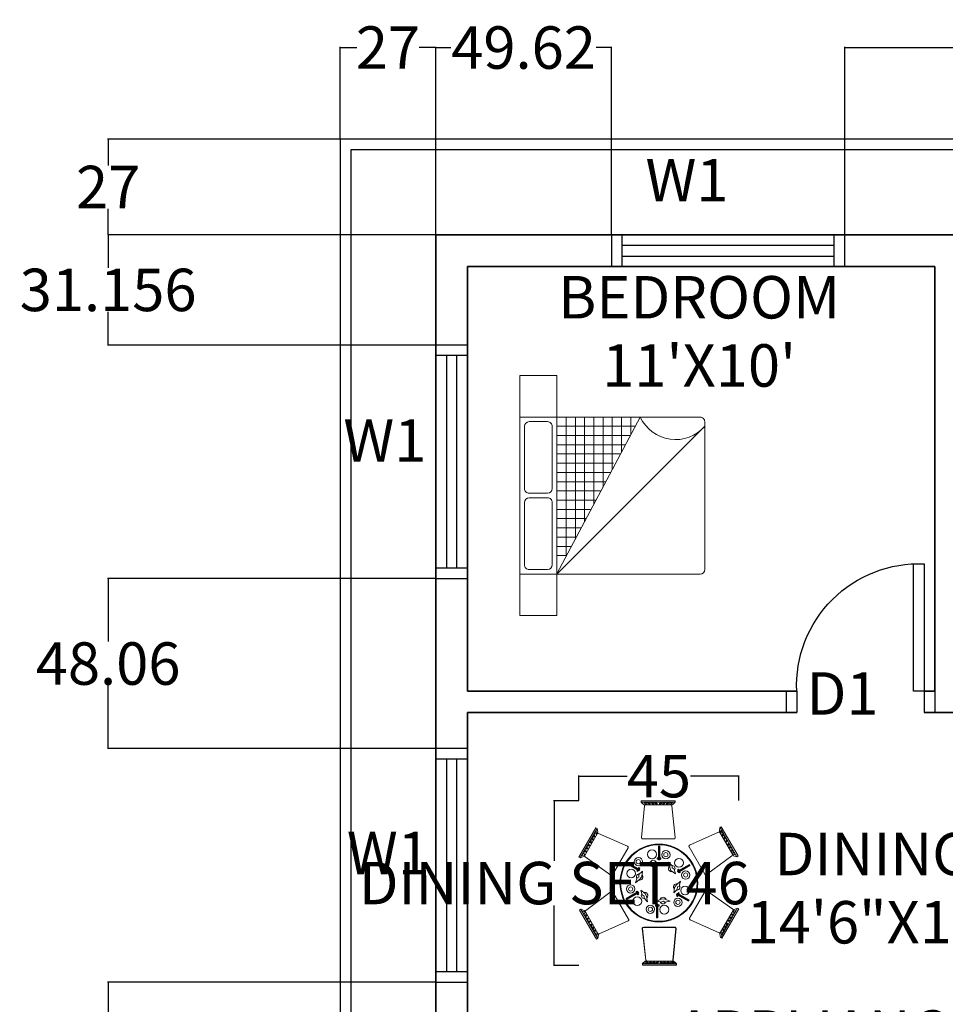
# Model space of a CAD drawing. Units: inches. Extents: x 774 to 1314, y 374 to 930.
# Tile 4 of 5: x 774 to 1035, y 652 to 930. Entities that reach past the tile are written whole.
import ezdxf
from ezdxf.enums import TextEntityAlignment as Align

# ---------------------------------------------------------------- set-up
doc = ezdxf.new("R2010")
doc.units = ezdxf.units.IN
doc.header["$MEASUREMENT"] = 0
for name, color, linetype, lineweight in [('A-ANNO-DIMS', 2, 'Continuous', 18), ('A-ANNO-TEXT', 2, 'Continuous', 18), ('A-AREA-IDEN', 2, 'Continuous', 18), ('A-DOOR', 6, 'Continuous', 25), ('A-FURN', 8, 'Continuous', 18), ('A-GLAZ', 4, 'Continuous', 18), ('A-WALL', 1, 'Continuous', 35), ('C-PROP', 3, 'Continuous', 25)]:
    doc.layers.add(name, color=color, linetype=linetype, lineweight=lineweight)
doc.layers.add('Layer4', color=4, linetype='Continuous')
doc.styles.get("Standard").update_dxf_attribs({"font": 'arial.ttf'})
doc.dimstyles.get("Standard").update_dxf_attribs({"dimtxt": 12, "dimasz": 0.18, "dimexe": 0.18, "dimexo": 0.0625, "dimgap": 0.09, "dimtad": 0, "dimtih": 1, "dimtoh": 1, "dimdec": 0, "dimzin": 0, "dimdsep": 46, "dimlunit": 4, "dimtxsty": 'Standard', "dimcen": 0.09, "dimadec": 0, "dimazin": 0, "dimtfac": 1, "dimtdec": 0, "dimtofl": 0, "dimtmove": 0, "dimatfit": 3, "dimfxl": 1, "dimtolj": 1, "dimtzin": 0, "dimarcsym": 0})

# ---------------------------------------------------------------- blocks, each defined once
blk = doc.blocks.new('tr')
at = {"layer": 'Layer4'}
for p, q in [((9, 66), (0, 66)), ((9, 63), (0, 63)), ((0, 63), (0, 3)), ((3, 63), (3, 3)), ((6, 3), (6, 63)), ((9, 3), (9, 63)), ((0, 3), (9, 3)), ((0, 0), (9, 0))]:
    blk.add_line(p, q, dxfattribs=at)
blk = doc.blocks.new('A$C45501D90')
for p, q in [((-242, 1134), (224, 1134)), ((-242, 1113), (-242, 1134)), ((224, 1113), (-242, 1113)), ((-242, 1111), (-202, 1079)), ((-204, 1106), (-166, 1108)), ((-169, 1081), (-204, 1106)), ((-166, 1108), (-167, 1086)), ((-156, 1110), (-132, 1086)), ((-119, 1086), (-143, 1108)), ((-143, 1108), (-134, 1108)), ((-134, 1108), (-122, 1098)), ((-122, 1098), (-119, 1102)), ((-119, 1102), (-118, 1087)), ((-108, 1110), (-84, 1086)), ((-71, 1086), (-95, 1108)), ((-95, 1108), (-86, 1108)), ((-86, 1108), (-75, 1098)), ((-75, 1098), (-71, 1102)), ((-71, 1102), (-70, 1087)), ((-60, 1110), (-36, 1086)), ((-23, 1086), (-47, 1108)), ((-47, 1108), (-38, 1108)), ((-38, 1108), (-27, 1098)), ((-27, 1098), (-23, 1102)), ((-23, 1102), (-22, 1087)), ((8, 1102), (7, 1087)), ((8, 1086), (32, 1108)), ((12, 1098), (8, 1102)), ((23, 1108), (12, 1098)), ((45, 1110), (21, 1086)), ((32, 1108), (23, 1108)), ((56, 1102), (55, 1087)), ((56, 1086), (80, 1108)), ((60, 1098), (56, 1102)), ((71, 1108), (60, 1098)), ((93, 1110), (69, 1086)), ((80, 1108), (71, 1108)), ((104, 1102), (103, 1087)), ((104, 1086), (128, 1108)), ((107, 1098), (104, 1102)), ((119, 1108), (107, 1098)), ((141, 1110), (117, 1086)), ((128, 1108), (119, 1108)), ((189, 1106), (151, 1108)), ((151, 1108), (152, 1086)), ((154, 1081), (189, 1106)), ((224, 1113), (187, 1079)), ((224, 1134), (224, 1113)), ((-197, 1062), (-239, 628)), ((-202, 1079), (-169, 1081)), ((162, 1076), (-181, 1076)), ((-132, 1086), (-119, 1086)), ((-84, 1086), (-71, 1086)), ((-36, 1086), (-23, 1086)), ((21, 1086), (8, 1086)), ((69, 1086), (56, 1086)), ((117, 1086), (104, 1086)), ((187, 1079), (154, 1081)), ((225, 628), (178, 1062)), ((-1103, 357), (-870, 761)), ((-852, 750), (-1085, 347)), ((-864, 717), (-884, 684)), ((-884, 684), (-864, 675)), ((-870, 761), (-852, 750)), ((-859, 674), (-864, 717)), ((-841, 702), (-859, 674)), ((-849, 752), (-841, 702)), ((-431, 509), (-831, 685)), ((821, 702), (424, 521)), ((841, 765), (834, 715)), ((834, 715), (852, 687)), ((1013, 398), (841, 695)), ((843, 766), (861, 776)), ((1076, 362), (843, 766)), ((852, 687), (856, 730)), ((856, 730), (877, 697)), ((877, 697), (857, 688)), ((861, 776), (1094, 373)), ((883, 690), (874, 657)), ((-851, 678), (-1023, 381)), ((-945, 559), (-950, 558)), ((-950, 558), (-938, 550)), ((-943, 582), (-948, 574)), ((-948, 574), (-945, 559)), ((-936, 550), (-943, 582)), ((-938, 594), (-930, 561)), ((-930, 561), (-936, 550)), ((-921, 601), (-926, 600)), ((-926, 600), (-914, 591)), ((-919, 624), (-924, 615)), ((-924, 615), (-921, 601)), ((-912, 592), (-919, 624)), ((-914, 635), (-906, 603)), ((-906, 603), (-912, 592)), ((-898, 642), (-902, 641)), ((-902, 641), (-890, 633)), ((-895, 665), (-900, 657)), ((-900, 657), (-898, 642)), ((-888, 633), (-895, 665)), ((-890, 677), (-882, 644)), ((-882, 644), (-888, 633)), ((-223, 610), (209, 610)), ((874, 657), (881, 646)), ((881, 646), (888, 678)), ((894, 654), (883, 646)), ((888, 678), (893, 670)), ((893, 670), (890, 655)), ((890, 655), (894, 654)), ((907, 648), (898, 616)), ((898, 616), (904, 605)), ((904, 605), (912, 637)), ((918, 613), (907, 604)), ((912, 637), (917, 628)), ((917, 628), (914, 614)), ((914, 614), (918, 613)), ((931, 607), (922, 574)), ((922, 574), (928, 563)), ((928, 563), (936, 595)), ((942, 571), (931, 563)), ((936, 595), (941, 587)), ((941, 587), (938, 572)), ((938, 572), (942, 571)), ((958, 543), (945, 538)), ((957, 539), (958, 543)), ((-1060, 377), (-1042, 411)), ((-1042, 411), (-1024, 398)), ((-1039, 420), (-1006, 428)), ((-1000, 440), (-1031, 430)), ((-1031, 430), (-1026, 438)), ((-1026, 438), (-1012, 443)), ((-1015, 461), (-982, 470)), ((-1012, 443), (-1014, 448)), ((-1014, 448), (-1000, 442)), ((-976, 481), (-1007, 471)), ((-1007, 471), (-1002, 480)), ((-1006, 428), (-1000, 440)), ((-1002, 480), (-989, 485)), ((-991, 503), (-958, 511)), ((-989, 485), (-990, 489)), ((-990, 489), (-976, 483)), ((-952, 522), (-983, 513)), ((-983, 513), (-978, 521)), ((-982, 470), (-976, 481)), ((-978, 521), (-965, 526)), ((-965, 526), (-966, 530)), ((-966, 530), (-953, 525)), ((-958, 511), (-952, 522)), ((-640, 112), (-424, 486)), ((-6, 509, 91), (0, 509, 91)), ((-6, 318, 91), (-6, 509, 91)), ((0, 509, 91), (0, 318, 91)), ((6, 318, 91), (6, 509, 91)), ((6, 509, 91), (12, 509, 91)), ((12, 509, 91), (12, 318, 91)), ((417, 498), (633, 124)), ((951, 524), (944, 535)), ((944, 535), (976, 526)), ((983, 516), (951, 524)), ((971, 534), (957, 539)), ((968, 494), (1000, 484)), ((975, 483), (968, 494)), ((982, 502), (969, 496)), ((976, 526), (971, 534)), ((1007, 474), (975, 483)), ((981, 498), (982, 502)), ((995, 493), (981, 498)), ((999, 441), (992, 453)), ((992, 453), (1024, 443)), ((1006, 461), (993, 455)), ((1000, 484), (995, 493)), ((1031, 433), (999, 441)), ((1005, 456), (1006, 461)), ((1019, 451), (1005, 456)), ((1035, 424), (1016, 411)), ((1024, 443), (1019, 451)), ((1053, 390), (1035, 424)), ((-1085, 347), (-1103, 357)), ((-1083, 346), (-1036, 364)), ((-1020, 394), (-1060, 377)), ((-1036, 364), (-1020, 394)), ((-1018, 360), (-663, 107)), ((-431, 275, 91), (-428, 280, 91)), ((-265, 180, 91), (-431, 275, 91)), ((-428, 280, 91), (-262, 185, 91)), ((-175, 276, 91), (-105, 293, 91)), ((-103, 252, 91), (-175, 276, 91)), ((-105, 293, 91), (-86, 278, 91)), ((-86, 278, 91), (-52, 294, 91)), ((9, 276, 91), (-60, 246, 91)), ((-52, 294, 91), (9, 276, 91)), ((-22, 329, 91), (-22, 345, 91)), ((-22, 345, 91), (-6, 345, 91)), ((-6, 329, 91), (-22, 329, 91)), ((0, 318, 91), (-6, 318, 91)), ((0, 345, 91), (6, 345, 91)), ((6, 329, 91), (0, 329, 91)), ((12, 318, 91), (6, 318, 91)), ((12, 345, 91), (27, 345, 91)), ((27, 329, 91), (12, 329, 91)), ((27, 345, 91), (27, 329, 91)), ((134, 288, 91), (184, 236, 91)), ((150, 214, 91), (134, 288, 91)), ((656, 119), (1008, 377)), ((1028, 377), (1013, 407)), ((1013, 407), (1053, 390)), ((1076, 359), (1028, 377)), ((1094, 373), (1076, 362)), ((-436, 265, 91), (-433, 271, 91)), ((-271, 170, 91), (-436, 265, 91)), ((-433, 271, 91), (-268, 175, 91)), ((-303, 169, 91), (-294, 183, 91)), ((-289, 161, 91), (-303, 169, 91)), ((-291, 188, 91), (-289, 193, 91)), ((-281, 176, 91), (-289, 161, 91)), ((-286, 198, 91), (-278, 212, 91)), ((-278, 212, 91), (-264, 204, 91)), ((-275, 185, 91), (-278, 181, 91)), ((-274, 118, 91), (-227, 162, 91)), ((-264, 204, 91), (-272, 191, 91)), ((-268, 175, 91), (-271, 170, 91)), ((-262, 185, 91), (-265, 180, 91)), ((-227, 162, 91), (-236, 87, 91)), ((-60, 246, 91), (-103, 252, 91)), ((166, 173, 91), (150, 214, 91)), ((227, 128, 91), (166, 173, 91)), ((184, 236, 91), (181, 211, 91)), ((181, 211, 91), (211, 190, 91)), ((211, 190, 91), (227, 128, 91)), ((255, 162, 91), (421, 257, 91)), ((258, 157, 91), (255, 162, 91)), ((257, 182, 91), (270, 190, 91)), ((265, 168, 91), (257, 182, 91)), ((424, 252, 91), (258, 157, 91)), ((261, 152, 91), (426, 248, 91)), ((264, 147, 91), (261, 152, 91)), ((429, 242, 91), (264, 147, 91)), ((271, 158, 91), (268, 162, 91)), ((270, 190, 91), (278, 175, 91)), ((281, 139, 91), (274, 153, 91)), ((281, 170, 91), (284, 165, 91)), ((295, 147, 91), (281, 139, 91)), ((287, 160, 91), (295, 147, 91)), ((421, 257, 91), (424, 252, 91)), ((426, 248, 91), (429, 242, 91)), ((-320, 2, 91), (-299, 72, 91)), ((-263, 53, 91), (-320, 2, 91)), ((-299, 72, 91), (-277, 81, 91)), ((-277, 81, 91), (-274, 118, 91)), ((-236, 87, 91), (-263, 53, 91)), ((243, -25, 91), (299, 26, 91)), ((299, 26, 91), (279, -44, 91)), ((-656, -119), (-1008, -377)), ((-417, -498), (-633, -124)), ((-450, -214, 91), (-284, -119, 91)), ((-281, -124, 91), (-447, -220, 91)), ((-444, -224, 91), (-279, -129, 91)), ((-276, -134, 91), (-441, -229, 91)), ((-315, -119, 91), (-302, -111, 91)), ((-307, -132, 91), (-315, -119, 91)), ((-302, -111, 91), (-294, -125, 91)), ((-291, -130, 91), (-288, -134, 91)), ((-284, -119, 91), (-281, -124, 91)), ((-279, -129, 91), (-276, -134, 91)), ((-247, -100, 91), (-187, -145, 91)), ((-232, -162, 91), (-247, -100, 91)), ((207, -134, 91), (216, -60, 91)), ((253, -90, 91), (207, -134, 91)), ((216, -60, 91), (243, -25, 91)), ((256, -53, 91), (253, -90, 91)), ((279, -44, 91), (256, -53, 91)), ((260, -148, 91), (269, -133, 91)), ((269, -133, 91), (282, -141, 91)), ((640, -112), (424, -486)), ((1018, -360), (663, -107)), ((-447, -220, 91), (-450, -214, 91)), ((-441, -229, 91), (-444, -224, 91)), ((-302, -142, 91), (-304, -137, 91)), ((-290, -162, 91), (-299, -147, 91)), ((-277, -154, 91), (-290, -162, 91)), ((-285, -140, 91), (-277, -154, 91)), ((-201, -183, 91), (-232, -162, 91)), ((-205, -208, 91), (-201, -183, 91)), ((-155, -260, 91), (-205, -208, 91)), ((-187, -145, 91), (-170, -186, 91)), ((-170, -186, 91), (-155, -260, 91)), ((-30, -248, 91), (39, -218, 91)), ((32, -266, 91), (-30, -248, 91)), ((65, -250, 91), (32, -266, 91)), ((39, -218, 91), (83, -224, 91)), ((84, -265, 91), (65, -250, 91)), ((83, -224, 91), (155, -248, 91)), ((155, -248, 91), (84, -265, 91)), ((242, -157, 91), (245, -152, 91)), ((407, -252, 91), (242, -157, 91)), ((244, -176, 91), (252, -163, 91)), ((257, -184, 91), (244, -176, 91)), ((245, -152, 91), (410, -247, 91)), ((248, -147, 91), (251, -142, 91)), ((413, -243, 91), (248, -147, 91)), ((251, -142, 91), (416, -237, 91)), ((255, -157, 91), (257, -153, 91)), ((265, -170, 91), (257, -184, 91)), ((271, -160, 91), (268, -165, 91)), ((282, -141, 91), (274, -155, 91)), ((410, -247, 91), (407, -252, 91)), ((416, -237, 91), (413, -243, 91)), ((-1094, -373), (-1076, -362)), ((-861, -776), (-1094, -373)), ((-1076, -359), (-1028, -377)), ((-1076, -362), (-843, -766)), ((-1053, -390), (-1035, -424)), ((-1013, -407), (-1053, -390)), ((-1028, -377), (-1013, -407)), ((-1013, -398), (-841, -695)), ((-48, -317, 91), (-48, -301, 91)), ((-48, -301, 91), (-32, -301, 91)), ((-32, -317, 91), (-48, -317, 91)), ((-32, -481, 91), (-32, -290, 91)), ((-32, -290, 91), (-26, -290, 91)), ((-26, -290, 91), (-26, -481, 91)), ((-26, -301, 91), (-21, -301, 91)), ((-21, -317, 91), (-26, -317, 91)), ((-21, -481, 91), (-21, -290, 91)), ((-21, -290, 91), (-15, -290, 91)), ((-15, -290, 91), (-15, -481, 91)), ((-15, -301, 91), (2, -301, 91)), ((2, -317, 91), (-15, -317, 91)), ((2, -301, 91), (2, -317, 91)), ((851, -678), (1023, -381)), ((852, -750), (1085, -347)), ((1103, -357), (870, -761)), ((1036, -364), (1020, -394)), ((1020, -394), (1060, -377)), ((1042, -411), (1024, -398)), ((1083, -346), (1036, -364)), ((1060, -377), (1042, -411)), ((1085, -347), (1103, -357)), ((-1035, -424), (-1016, -411)), ((-1031, -433), (-999, -441)), ((-1024, -443), (-1019, -451)), ((-992, -453), (-1024, -443)), ((-1019, -451), (-1005, -456)), ((-1007, -474), (-975, -483)), ((-1006, -461), (-993, -455)), ((-1005, -456), (-1006, -461)), ((-968, -494), (-1000, -484)), ((-1000, -484), (-995, -493)), ((-999, -441), (-992, -453)), ((-995, -493), (-981, -498)), ((-983, -516), (-951, -524)), ((-982, -502), (-969, -496)), ((-981, -498), (-982, -502)), ((-944, -535), (-976, -526)), ((-976, -526), (-971, -534)), ((-975, -483), (-968, -494)), ((-971, -534), (-957, -539)), ((-958, -543), (-945, -538)), ((-957, -539), (-958, -543)), ((-951, -524), (-944, -535)), ((-821, -702), (-424, -521)), ((-26, -481, 91), (-32, -481, 91)), ((-15, -481, 91), (-21, -481, 91)), ((431, -509), (831, -685)), ((958, -511), (952, -522)), ((952, -522), (983, -513)), ((966, -530), (953, -525)), ((991, -503), (958, -511)), ((978, -521), (965, -526)), ((965, -526), (966, -530)), ((982, -470), (976, -481)), ((976, -481), (1007, -471)), ((990, -489), (976, -483)), ((983, -513), (978, -521)), ((1015, -461), (982, -470)), ((1002, -480), (989, -485)), ((989, -485), (990, -489)), ((1006, -428), (1000, -440)), ((1000, -440), (1031, -430)), ((1014, -448), (1000, -442)), ((1007, -471), (1002, -480)), ((1039, -420), (1006, -428)), ((1026, -438), (1012, -443)), ((1012, -443), (1014, -448)), ((1031, -430), (1026, -438)), ((-942, -571), (-931, -563)), ((-938, -572), (-942, -571)), ((-941, -587), (-938, -572)), ((-936, -595), (-941, -587)), ((-928, -563), (-936, -595)), ((-931, -607), (-922, -574)), ((-922, -574), (-928, -563)), ((-918, -613), (-907, -604)), ((-914, -614), (-918, -613)), ((-917, -628), (-914, -614)), ((-912, -637), (-917, -628)), ((-904, -605), (-912, -637)), ((-907, -648), (-898, -616)), ((-898, -616), (-904, -605)), ((-894, -654), (-883, -646)), ((-890, -655), (-894, -654)), ((-893, -670), (-890, -655)), ((-888, -678), (-893, -670)), ((-881, -646), (-888, -678)), ((-883, -690), (-874, -657)), ((-874, -657), (-881, -646)), ((-229, -629), (-182, -1063)), ((-225, -628), (-178, -1062)), ((219, -612), (-213, -612)), ((223, -610), (-209, -610)), ((193, -1063), (235, -629)), ((197, -1062), (239, -628)), ((841, -702), (859, -674)), ((859, -674), (864, -717)), ((884, -684), (864, -675)), ((882, -644), (888, -633)), ((890, -677), (882, -644)), ((888, -633), (895, -665)), ((902, -641), (890, -633)), ((895, -665), (900, -657)), ((898, -642), (902, -641)), ((900, -657), (898, -642)), ((906, -603), (912, -592)), ((914, -635), (906, -603)), ((912, -592), (919, -624)), ((926, -600), (914, -591)), ((919, -624), (924, -615)), ((921, -601), (926, -600)), ((924, -615), (921, -601)), ((930, -561), (936, -550)), ((938, -594), (930, -561)), ((936, -550), (943, -582)), ((950, -558), (938, -550)), ((943, -582), (948, -574)), ((945, -559), (950, -558)), ((948, -574), (945, -559)), ((-877, -697), (-857, -688)), ((-856, -730), (-877, -697)), ((-843, -766), (-861, -776)), ((-852, -687), (-856, -730)), ((-834, -715), (-852, -687)), ((-841, -765), (-834, -715)), ((849, -752), (841, -702)), ((870, -761), (852, -750)), ((864, -717), (884, -684)), ((-231, -1113), (-191, -1081)), ((-227, -1111), (-187, -1079)), ((-158, -1082), (-193, -1108)), ((-191, -1081), (-158, -1082)), ((-154, -1081), (-189, -1106)), ((-187, -1079), (-154, -1081)), ((-166, -1078), (177, -1078)), ((-162, -1076), (181, -1076)), ((-151, -1108), (-152, -1086)), ((-141, -1110), (-117, -1086)), ((-104, -1086), (-128, -1108)), ((-117, -1086), (-104, -1086)), ((-93, -1110), (-69, -1086)), ((-56, -1086), (-80, -1108)), ((-69, -1086), (-56, -1086)), ((-45, -1110), (-21, -1086)), ((-8, -1086), (-32, -1108)), ((-21, -1086), (-8, -1086)), ((23, -1086), (47, -1108)), ((36, -1086), (23, -1086)), ((60, -1110), (36, -1086)), ((71, -1086), (95, -1108)), ((84, -1086), (71, -1086)), ((108, -1110), (84, -1086)), ((119, -1086), (143, -1108)), ((132, -1086), (119, -1086)), ((156, -1110), (132, -1086)), ((198, -1081), (165, -1082)), ((165, -1082), (200, -1108)), ((166, -1108), (167, -1086)), ((202, -1079), (169, -1081)), ((169, -1081), (204, -1106)), ((238, -1113), (198, -1081)), ((242, -1111), (202, -1079)), ((-228, -1114), (238, -1114)), ((-228, -1135), (-228, -1114)), ((238, -1135), (-228, -1135)), ((-224, -1113), (242, -1113)), ((-224, -1134), (-224, -1113)), ((242, -1134), (-224, -1134)), ((-193, -1108), (-155, -1109)), ((-189, -1106), (-151, -1108)), ((-155, -1109), (-156, -1087)), ((-145, -1111), (-121, -1087)), ((-108, -1087), (-132, -1109)), ((-132, -1109), (-123, -1109)), ((-128, -1108), (-119, -1108)), ((-123, -1109), (-112, -1100)), ((-121, -1087), (-108, -1087)), ((-119, -1108), (-107, -1098)), ((-112, -1100), (-108, -1103)), ((-108, -1103), (-107, -1089)), ((-107, -1098), (-104, -1102)), ((-104, -1102), (-103, -1087)), ((-97, -1111), (-73, -1087)), ((-60, -1087), (-84, -1109)), ((-84, -1109), (-75, -1109)), ((-80, -1108), (-71, -1108)), ((-75, -1109), (-64, -1100)), ((-73, -1087), (-60, -1087)), ((-71, -1108), (-60, -1098)), ((-64, -1100), (-60, -1103)), ((-60, -1103), (-59, -1089)), ((-60, -1098), (-56, -1102)), ((-56, -1102), (-55, -1087)), ((-49, -1111), (-25, -1087)), ((-13, -1087), (-37, -1109)), ((-37, -1109), (-27, -1109)), ((-32, -1108), (-23, -1108)), ((-27, -1109), (-16, -1100)), ((-25, -1087), (-13, -1087)), ((-23, -1108), (-12, -1098)), ((-16, -1100), (-13, -1103)), ((-13, -1103), (-11, -1089)), ((-12, -1098), (-8, -1102)), ((-8, -1102), (-7, -1087)), ((19, -1103), (18, -1089)), ((19, -1087), (43, -1109)), ((32, -1087), (19, -1087)), ((23, -1100), (19, -1103)), ((23, -1102), (22, -1087)), ((27, -1098), (23, -1102)), ((34, -1109), (23, -1100)), ((38, -1108), (27, -1098)), ((56, -1111), (32, -1087)), ((43, -1109), (34, -1109)), ((47, -1108), (38, -1108)), ((67, -1103), (66, -1089)), ((67, -1087), (91, -1109)), ((80, -1087), (67, -1087)), ((70, -1100), (67, -1103)), ((71, -1102), (70, -1087)), ((82, -1109), (70, -1100)), ((75, -1098), (71, -1102)), ((86, -1108), (75, -1098)), ((104, -1111), (80, -1087)), ((91, -1109), (82, -1109)), ((95, -1108), (86, -1108)), ((115, -1103), (114, -1089)), ((115, -1087), (139, -1109)), ((128, -1087), (115, -1087)), ((118, -1100), (115, -1103)), ((119, -1102), (118, -1087)), ((130, -1109), (118, -1100)), ((122, -1098), (119, -1102)), ((134, -1108), (122, -1098)), ((152, -1111), (128, -1087)), ((139, -1109), (130, -1109)), ((143, -1108), (134, -1108)), ((161, -1109), (163, -1087)), ((200, -1108), (161, -1109)), ((204, -1106), (166, -1108)), ((238, -1114), (238, -1135)), ((242, -1113), (242, -1134))]:
    blk.add_line(p, q)
for centre, radius in [((0, 0), 537), ((0, 0), 527), ((-95, 395, 91), 61.3), ((97, 390, 91), 56.9), ((96, 391, 91), 29.4), ((-282, 295, 91), 56.9), ((-284, 294, 91), 29.4), ((277, 278, 91), 61.3), ((-382, 131, 91), 61.3), ((369, 109, 91), 56.9), ((369, 111, 91), 29.4), ((-389, -81, 91), 56.9), ((-389, -83, 91), 29.4), ((362, -103, 91), 61.3), ((-298, -250, 91), 61.3), ((262, -267, 91), 56.9), ((263, -266, 91), 29.4), ((-117, -362, 91), 56.9), ((-116, -363, 91), 29.4), ((74, -367, 91), 61.3)]:
    blk.add_circle(centre, radius)
for centre, radius, start, end in [((-181, 1060), 16, 90, 174.5199), ((162, 1060), 16, 6.2572, 90), ((-837, 670), 16, 66.2572, 150), ((827, 687), 16, 30, 114.5199), ((-223, 626), 16, 174.5199, 270), ((209, 626), 16, 270, 6.2572), ((-438, 494), 16, 330, 66.2572), ((431, 506), 16, 114.5199, 210), ((-1009, 373), 16, 150, 234.5199), ((-77, 270, 91), 44.6, 25.8558, 153.3359), ((999, 390), 16, 306.2572, 30), ((-77, 270, 91), 44.6, 195.9338, 342.9389), ((178, 200, 91), 44.6, 135.9338, 282.9389), ((178, 200, 91), 44.6, 325.8558, 93.3359), ((-654, 120), 16, 234.5199, 330), ((-266, 84, 91), 44.6, 85.8558, 213.3359), ((-266, 84, 91), 44.6, 255.9338, 42.9389), ((647, 132), 16, 210, 306.2572), ((-647, -132), 16, 30, 126.2572), ((-198, -172, 91), 44.6, 315.9338, 102.9389), ((245, -56, 91), 44.6, 75.9338, 222.9389), ((245, -56, 91), 44.6, 265.8558, 33.3359), ((654, -120), 16, 54.5199, 150), ((-198, -172, 91), 44.6, 145.8558, 273.3359), ((57, -242, 91), 44.6, 15.9338, 162.9389), ((57, -242, 91), 44.6, 205.8558, 333.3359), ((-999, -390), 16, 126.2572, 210), ((1009, -373), 16, 330, 54.5199), ((-431, -506), 16, 294.5199, 30), ((438, -494), 16, 150, 246.2572), ((-213, -628), 16, 90, 186.2572), ((-209, -626), 16, 90, 186.2572), ((219, -628), 16, 354.5199, 90), ((223, -626), 16, 354.5199, 90), ((837, -670), 16, 246.2572, 330), ((-827, -687), 16, 210, 294.5199), ((-166, -1062), 16, 186.2572, 270), ((-162, -1060), 16, 186.2572, 270), ((177, -1062), 16, 270, 354.5199), ((181, -1060), 16, 270, 354.5199)]:
    blk.add_arc(centre, radius, start, end)
blk = doc.blocks.new('A$C4CBC1980')
for p, q in [((0.45, 2), (0, 2)), ((0, 2), (0, 1.6)), ((0, 2), (2.6, 2)), ((2.15, 2), (0.45, 2)), ((0.45, 2), (0.45, 0.05)), ((0.45, 0.05), (0.45, 2)), ((1.225, 1.95), (0.55, 1.95)), ((2.05, 1.95), (1.375, 1.95)), ((2.6, 2), (2.025, 2)), ((2.15, 0.05), (2.15, 2)), ((2.6, 1.6), (2.6, 2)), ((0.5, 1.9), (0.5, 1.7)), ((1.275, 1.7), (1.275, 1.9)), ((1.325, 1.7), (1.325, 1.9)), ((2.1, 1.7), (2.1, 1.9)), ((2.6, 1.6), (0, 1.6)), ((0.45, 1.6), (2.05, 0)), ((0.451, 1.6), (2.15, 0.697)), ((1.225, 1.65), (0.55, 1.65)), ((2.15, 1.6), (0.587, 1.6)), ((0.65, 1.494), (0.65, 1.6)), ((0.75, 1.441), (0.75, 1.6)), ((0.85, 1.388), (0.85, 1.6)), ((0.95, 1.335), (0.95, 1.6)), ((1.05, 1.282), (1.05, 1.6)), ((1.15, 1.229), (1.15, 1.6)), ((1.25, 1.176), (1.25, 1.6)), ((1.35, 1.122), (1.35, 1.6)), ((2.05, 1.65), (1.375, 1.65)), ((1.45, 1.069), (1.45, 1.6)), ((1.55, 1.016), (1.55, 1.6)), ((1.65, 0.986), (1.65, 1.6)), ((1.75, 0.91), (1.75, 1.6)), ((1.85, 0.857), (1.85, 1.6)), ((1.95, 0.804), (1.95, 1.6)), ((2.05, 0.751), (2.05, 1.6)), ((2.15, 1.5), (0.639, 1.5)), ((2.15, 1.4), (0.827, 1.4)), ((2.15, 1.3), (1.016, 1.3)), ((2.15, 1.2), (1.204, 1.2)), ((2.15, 1.1), (1.392, 1.1)), ((2.15, 1), (1.58, 1)), ((2.15, 0.9), (1.769, 0.9)), ((2.15, 0.8), (1.957, 0.8)), ((0.5, 0), (2.1, 0))]:
    blk.add_line(p, q)
for centre, radius, start, end in [((0.55, 1.9), 0.05, 90, 180), ((1.225, 1.9), 0.05, 0, 90), ((1.375, 1.9), 0.05, 90, 180), ((2.05, 1.9), 0.05, 0, 90), ((0.55, 1.7), 0.05, 180, 270), ((1.225, 1.7), 0.05, 270, 0), ((1.375, 1.7), 0.05, 180, 270), ((2.05, 1.7), 0.05, 270, 0), ((2.327, 0.316), 0.421, 114.9633, 228.7161), ((0.5, 0.05), 0.05, 180, 270), ((0.5, 0.05), 0.05, 180, 270), ((2.1, 0.05), 0.05, 270, 0)]:
    blk.add_arc(centre, radius, start, end)
blk = doc.blocks.new('DOOR-SWING-36IN')
blk.add_lwpolyline([(0, 0), (3, 0), (3, 36), (0, 36)], close=True)
blk.add_arc((1.5, 1.5), 34.53, 357.5104, 92.4896)
blk = doc.blocks.new('*D41')
at = {"layer": 'A-ANNO-DIMS', "color": 0, "lineweight": -2, "transparency": 16777216}
for p, q in [((931.72, 709.58), (924.63, 709.58)), ((924.81, 709.4), (924.81, 692.63)), ((924.81, 663.26), (924.81, 680.04)), ((931.72, 663.08), (924.63, 663.08))]:
    blk.add_line(p, q, dxfattribs=at)
at = {"layer": 'A-ANNO-DIMS', "color": 0, "transparency": 16777216}
for points in [[(924.78, 709.4), (924.84, 709.4), (924.81, 709.58)], [(924.78, 663.26), (924.84, 663.26), (924.81, 663.08)]]:
    blk.add_solid(points, dxfattribs=at)
at = {"layer": 'Defpoints', "color": 0, "transparency": 16777216}
for p in [(924.81, 709.58), (931.78, 709.58), (931.78, 663.08)]:
    blk.add_point(p, dxfattribs=at)
at = {"layer": 'A-ANNO-DIMS', "color": 0, "transparency": 16777216, "insert": (924.81, 686.33), "char_height": 12, "attachment_point": 5}
blk.add_mtext('\\A1;DINING SET 46', dxfattribs=at)
blk = doc.blocks.new('*D42')
at = {"layer": 'A-ANNO-DIMS', "color": 0, "lineweight": -2, "transparency": 16777216}
for p, q in [((931.78, 709.65), (931.78, 716.74)), ((931.96, 716.56), (945.41, 716.56)), ((976.81, 716.56), (963.36, 716.56)), ((976.99, 709.65), (976.99, 716.74))]:
    blk.add_line(p, q, dxfattribs=at)
at = {"layer": 'A-ANNO-DIMS', "color": 0, "transparency": 16777216}
for points in [[(931.96, 716.59), (931.96, 716.53), (931.78, 716.56)], [(976.81, 716.59), (976.81, 716.53), (976.99, 716.56)]]:
    blk.add_solid(points, dxfattribs=at)
at = {"layer": 'Defpoints', "color": 0, "transparency": 16777216}
for p in [(976.99, 716.56), (931.78, 709.58), (976.99, 709.58)]:
    blk.add_point(p, dxfattribs=at)
at = {"layer": 'A-ANNO-DIMS', "color": 0, "transparency": 16777216, "insert": (954.39, 716.56), "char_height": 12, "attachment_point": 5}
blk.add_mtext('\\A1;45', dxfattribs=at)
blk = doc.blocks.new('*D51')
at = {"layer": 'A-ANNO-DIMS', "color": 0, "lineweight": -2, "transparency": 16777216}
for p, q in [((1072.03, 644.35), (1071.85, 644.35)), ((1072.03, 640.32), (1072.03, 644.53)), ((1099.12, 644.35), (1072.21, 644.35)), ((1099.3, 640.32), (1099.3, 644.53))]:
    blk.add_line(p, q, dxfattribs=at)
at = {"layer": 'A-ANNO-DIMS', "color": 0, "transparency": 16777216}
for points in [[(1072.21, 644.38), (1072.21, 644.32), (1072.03, 644.35)], [(1099.12, 644.38), (1099.12, 644.32), (1099.3, 644.35)]]:
    blk.add_solid(points, dxfattribs=at)
at = {"layer": 'Defpoints', "color": 0, "transparency": 16777216}
for p in [(1072.03, 644.35), (1072.03, 640.25), (1099.3, 640.25)]:
    blk.add_point(p, dxfattribs=at)
at = {"layer": 'A-ANNO-DIMS', "color": 0, "transparency": 16777216, "insert": (1013.43, 644.35), "char_height": 12, "attachment_point": 5}
blk.add_mtext('\\A1;APPLIANCE 27', dxfattribs=at)
blk = doc.blocks.new('*D55')
at = {"layer": 'A-ANNO-DIMS', "color": 0, "lineweight": -2, "transparency": 16777216}
for p, q in [((864.33, 896.63), (864.33, 922.67)), ((864.51, 922.49), (869.05, 922.49)), ((891.15, 922.49), (886.62, 922.49)), ((891.33, 869.63), (891.33, 922.67))]:
    blk.add_line(p, q, dxfattribs=at)
at = {"layer": 'A-ANNO-DIMS', "color": 0, "transparency": 16777216}
for points in [[(864.51, 922.52), (864.51, 922.46), (864.33, 922.49)], [(891.15, 922.52), (891.15, 922.46), (891.33, 922.49)]]:
    blk.add_solid(points, dxfattribs=at)
at = {"layer": 'Defpoints', "color": 0, "transparency": 16777216}
for p in [(891.33, 922.49), (864.33, 896.57), (891.33, 869.57)]:
    blk.add_point(p, dxfattribs=at)
at = {"layer": 'A-ANNO-DIMS', "color": 0, "transparency": 16777216, "insert": (877.83, 922.49), "char_height": 12, "attachment_point": 5}
blk.add_mtext('\\A1;27', dxfattribs=at)
blk = doc.blocks.new('*D56')
at = {"layer": 'A-ANNO-DIMS', "color": 0, "lineweight": -2, "transparency": 16777216}
for p, q in [((891.33, 869.63), (891.33, 922.67)), ((891.51, 922.49), (895.63, 922.49)), ((940.78, 922.49), (936.66, 922.49)), ((940.96, 869.63), (940.96, 922.67))]:
    blk.add_line(p, q, dxfattribs=at)
at = {"layer": 'A-ANNO-DIMS', "color": 0, "transparency": 16777216}
for points in [[(891.51, 922.52), (891.51, 922.46), (891.33, 922.49)], [(940.78, 922.52), (940.78, 922.46), (940.96, 922.49)]]:
    blk.add_solid(points, dxfattribs=at)
at = {"layer": 'Defpoints', "color": 0, "transparency": 16777216}
for p in [(940.96, 922.49), (891.33, 869.57), (940.96, 869.57)]:
    blk.add_point(p, dxfattribs=at)
at = {"layer": 'A-ANNO-DIMS', "color": 0, "transparency": 16777216, "insert": (916.15, 922.49), "char_height": 12, "attachment_point": 5}
blk.add_mtext('\\A1;49.62', dxfattribs=at)
blk = doc.blocks.new('*D57')
at = {"layer": 'A-ANNO-DIMS', "color": 0, "lineweight": -2, "transparency": 16777216}
for p, q in [((1006.96, 869.63), (1006.96, 922.67)), ((1007.14, 922.49), (1046.52, 922.49)), ((1046.7, 869.63), (1046.7, 922.67)), ((1046.7, 922.49), (1046.88, 922.49))]:
    blk.add_line(p, q, dxfattribs=at)
at = {"layer": 'A-ANNO-DIMS', "color": 0, "transparency": 16777216}
for points in [[(1007.14, 922.52), (1007.14, 922.46), (1006.96, 922.49)], [(1046.52, 922.52), (1046.52, 922.46), (1046.7, 922.49)]]:
    blk.add_solid(points, dxfattribs=at)
at = {"layer": 'Defpoints', "color": 0, "transparency": 16777216}
for p in [(1046.7, 922.49), (1006.96, 869.57), (1046.7, 869.57)]:
    blk.add_point(p, dxfattribs=at)
at = {"layer": 'A-ANNO-DIMS', "color": 0, "transparency": 16777216, "insert": (1071.85, 922.49), "char_height": 12, "attachment_point": 5}
blk.add_mtext('\\A1;39.744', dxfattribs=at)
blk = doc.blocks.new('*D63')
at = {"layer": 'A-ANNO-DIMS', "color": 0, "lineweight": -2, "transparency": 16777216}
for p, q in [((891.27, 658.35), (798.56, 658.35)), ((798.74, 658.17), (798.74, 647.34)), ((798.74, 624.06), (798.74, 634.89)), ((891.27, 623.88), (798.56, 623.88))]:
    blk.add_line(p, q, dxfattribs=at)
at = {"layer": 'A-ANNO-DIMS', "color": 0, "transparency": 16777216}
for points in [[(798.71, 658.17), (798.77, 658.17), (798.74, 658.35)], [(798.71, 624.06), (798.77, 624.06), (798.74, 623.88)]]:
    blk.add_solid(points, dxfattribs=at)
at = {"layer": 'Defpoints', "color": 0, "transparency": 16777216}
for p in [(798.74, 658.35), (891.33, 658.35), (891.33, 623.88)]:
    blk.add_point(p, dxfattribs=at)
at = {"layer": 'A-ANNO-DIMS', "color": 0, "transparency": 16777216, "insert": (798.74, 641.11), "char_height": 12, "attachment_point": 5}
blk.add_mtext('\\A1;34.465', dxfattribs=at)
blk = doc.blocks.new('*D64')
at = {"layer": 'A-ANNO-DIMS', "color": 0, "lineweight": -2, "transparency": 16777216}
for p, q in [((891.27, 772.41), (798.56, 772.41)), ((798.74, 772.23), (798.74, 754.6)), ((798.74, 724.53), (798.74, 742.16)), ((891.27, 724.35), (798.56, 724.35))]:
    blk.add_line(p, q, dxfattribs=at)
at = {"layer": 'A-ANNO-DIMS', "color": 0, "transparency": 16777216}
for points in [[(798.71, 772.23), (798.77, 772.23), (798.74, 772.41)], [(798.71, 724.53), (798.77, 724.53), (798.74, 724.35)]]:
    blk.add_solid(points, dxfattribs=at)
at = {"layer": 'Defpoints', "color": 0, "transparency": 16777216}
for p in [(798.74, 772.41), (891.33, 772.41), (891.33, 724.35)]:
    blk.add_point(p, dxfattribs=at)
at = {"layer": 'A-ANNO-DIMS', "color": 0, "transparency": 16777216, "insert": (798.74, 748.38), "char_height": 12, "attachment_point": 5}
blk.add_mtext('\\A1;48.06', dxfattribs=at)
blk = doc.blocks.new('*D65')
at = {"layer": 'A-ANNO-DIMS', "color": 0, "lineweight": -2, "transparency": 16777216}
for p, q in [((891.27, 869.57), (798.56, 869.57)), ((798.74, 869.39), (798.74, 860.21)), ((798.74, 838.59), (798.74, 847.77)), ((891.27, 838.41), (798.56, 838.41))]:
    blk.add_line(p, q, dxfattribs=at)
at = {"layer": 'A-ANNO-DIMS', "color": 0, "transparency": 16777216}
for points in [[(798.71, 869.39), (798.77, 869.39), (798.74, 869.57)], [(798.71, 838.59), (798.77, 838.59), (798.74, 838.41)]]:
    blk.add_solid(points, dxfattribs=at)
at = {"layer": 'Defpoints', "color": 0, "transparency": 16777216}
for p in [(798.74, 869.57), (891.33, 869.57), (891.33, 838.41)]:
    blk.add_point(p, dxfattribs=at)
at = {"layer": 'A-ANNO-DIMS', "color": 0, "transparency": 16777216, "insert": (798.74, 853.99), "char_height": 12, "attachment_point": 5}
blk.add_mtext('\\A1;31.156', dxfattribs=at)
blk = doc.blocks.new('*D66')
at = {"layer": 'A-ANNO-DIMS', "color": 0, "lineweight": -2, "transparency": 16777216}
for p, q in [((864.27, 896.57), (798.56, 896.57)), ((798.74, 896.39), (798.74, 889.18)), ((798.74, 869.75), (798.74, 876.95)), ((891.27, 869.57), (798.56, 869.57))]:
    blk.add_line(p, q, dxfattribs=at)
at = {"layer": 'A-ANNO-DIMS', "color": 0, "transparency": 16777216}
for points in [[(798.71, 896.39), (798.77, 896.39), (798.74, 896.57)], [(798.71, 869.75), (798.77, 869.75), (798.74, 869.57)]]:
    blk.add_solid(points, dxfattribs=at)
at = {"layer": 'Defpoints', "color": 0, "transparency": 16777216}
for p in [(798.74, 896.57), (864.33, 896.57), (891.33, 869.57)]:
    blk.add_point(p, dxfattribs=at)
at = {"layer": 'A-ANNO-DIMS', "color": 0, "transparency": 16777216, "insert": (798.74, 883.07), "char_height": 12, "attachment_point": 5}
blk.add_mtext('\\A1;27', dxfattribs=at)

msp = doc.modelspace()

# ---------------------------------------------------------------- linework, layer by layer
at = {"layer": 'A-DOOR'}
for p, q in [((990.3347, 740.5656), (990.3347, 734.5656)), ((993.3347, 740.5656), (993.3347, 734.5656)), ((1029.3347, 740.5656), (1029.3347, 734.5656)), ((1032.3347, 740.5656), (1032.3347, 734.5656))]:
    msp.add_line(p, q, dxfattribs=at)
at = {"layer": 'A-WALL'}
for p, q in [((900.3347, 860.5656), (900.3347, 740.5656)), ((1032.3347, 860.5656), (900.3347, 860.5656)), ((1032.3347, 860.5656), (1032.3347, 740.5656)), ((993.3347, 740.5656), (900.3347, 740.5656)), ((1032.3347, 740.5656), (1029.3347, 740.5656)), ((900.3347, 734.5656), (900.3347, 536.5656)), ((993.3347, 734.5656), (900.3347, 734.5656)), ((1038.3347, 734.5656), (1029.3347, 734.5656))]:
    msp.add_line(p, q, dxfattribs=at)
msp.add_lwpolyline([(1203.3347, 740.5656), (1203.3347, 869.5656), (891.3347, 869.5656), (891.3347, 527.5656)], dxfattribs=at)
at = {"layer": 'C-PROP'}
msp.add_lwpolyline([(864.3347, 410.5656), (1230.3347, 410.5656), (1230.3347, 896.5656), (864.3347, 896.5656)], close=True, dxfattribs=at)
msp.add_lwpolyline([(1227.3347, 740.5656), (1227.3347, 893.5656), (867.3347, 893.5656), (867.3347, 413.5656), (975.3347, 413.5656)], dxfattribs=at)

# ---------------------------------------------------------------- block references
at = {"layer": 'A-DOOR', "extrusion": (0, 0, -1), "zscale": -1}
msp.add_blockref('DOOR-SWING-36IN', (-1029.3344, 740.566), dxfattribs=at)
at = {"layer": 'A-FURN', "xscale": 26.11182411513011, "yscale": 26.11182411513011, "zscale": 26.11182411513011, "rotation": 89.99999999999999}
msp.add_blockref('A$C4CBC1980', (967.3427, 761.9155), dxfattribs=at)
at = {"layer": 'A-FURN', "xscale": 0.0204978781153701, "yscale": 0.0204978781153701, "zscale": 0.0204978781153701}
msp.add_blockref('A$C45501D90', (954.3862, 686.3485, 88.906), dxfattribs=at)
at = {"layer": 'A-GLAZ', "rotation": 270}
msp.add_blockref('tr', (940.9565, 869.5656), dxfattribs=at)
at = {"layer": 'A-GLAZ'}
for p in [(891.3347, 772.4101), (891.3347, 658.3472)]:
    msp.add_blockref('tr', p, dxfattribs=at)

# ---------------------------------------------------------------- texts
at = {"layer": 'A-ANNO-TEXT'}
for s, p in [('W1', (962.3405, 878.9863)), ('W1', (876.9516, 805.4031)), ('D1', (1006.3027, 733.9204)), ('W1', (877.9489, 688.8175))]:
    msp.add_text(s, height=12, dxfattribs=at).set_placement(p, align=Align.CENTER)
at = {"layer": 'A-AREA-IDEN'}
for s, p in [('BEDROOM', (965.7741, 845.9101)), ("11'X10'", (965.7741, 826.6331)), ('DINING', (1015.004, 688.5358)), ('14\'6"X10\'', (1015.004, 669.2588))]:
    msp.add_text(s, height=12, dxfattribs=at).set_placement(p, align=Align.CENTER)

# ---------------------------------------------------------------- dimensions: what is measured, and where the dimension line sits
at = {"layer": 'A-ANNO-DIMS'}
for base, p1, p2, override, picture, middle in [((891.3347, 922.4906), (864.3347, 896.5656), (891.3347, 869.5656), {"dimdec": 0, "dimlfac": 1, "dimrnd": 0, "dimzin": 0, "dimdsep": 46, "dimlunit": 2}, '*D55', (877.8347, 922.4906)), ((940.9565, 922.4906), (891.3347, 869.5656), (940.9565, 869.5656), {"dimdec": 2, "dimlfac": 1, "dimrnd": 0, "dimzin": 0, "dimdsep": 46, "dimlunit": 2}, '*D56', (916.1456, 922.4906)), ((1046.7007, 922.4906), (1006.9565, 869.5656), (1046.7007, 869.5656), {"dimdec": 3, "dimlfac": 1, "dimrnd": 0, "dimzin": 0, "dimdsep": 46, "dimlunit": 2}, '*D57', (1071.8506, 922.4906)), ((976.99, 716.5578), (931.7824, 709.5828), (976.99, 709.5828), {"dimdec": 0, "dimlfac": 1, "dimrnd": 0, "dimzin": 0, "dimdsep": 46, "dimlunit": 2}, '*D42', (954.3862, 716.5578))]:
    dim = msp.add_linear_dim(base=base, p1=p1, p2=p2, dimstyle='Standard', override=override, dxfattribs=at)
    dim.commit()
    dim.dimension.update_dxf_attribs({"geometry": picture, "text_midpoint": middle})
for base, p1, p2, override, picture, middle in [((798.7384, 896.5656), (891.3347, 869.5656), (864.3347, 896.5656), {"dimdec": 0, "dimlfac": 1, "dimrnd": 0, "dimzin": 0, "dimdsep": 46, "dimlunit": 2}, '*D66', (798.7384, 883.0656)), ((798.73836, 869.5656), (891.3347, 838.41006), (891.3347, 869.5656), {"dimdec": 3, "dimlfac": 1, "dimrnd": 0, "dimzin": 0, "dimdsep": 46, "dimlunit": 2}, '*D65', (798.73836, 853.98783)), ((798.7384, 772.4101), (891.3347, 724.3472), (891.3347, 772.4101), {"dimdec": 2, "dimlfac": 1, "dimrnd": 0, "dimzin": 0, "dimdsep": 46, "dimlunit": 2}, '*D64', (798.7384, 748.3786)), ((798.7384, 658.3472), (891.3347, 623.8818), (891.3347, 658.3472), {"dimdec": 3, "dimlfac": 1, "dimrnd": 0, "dimzin": 0, "dimdsep": 46, "dimlunit": 2}, '*D63', (798.7384, 641.1145))]:
    dim = msp.add_linear_dim(base=base, p1=p1, p2=p2, angle=90, dimstyle='Standard', override=override, dxfattribs=at)
    dim.commit()
    dim.dimension.update_dxf_attribs({"geometry": picture, "text_midpoint": middle})
for base, p1, p2, angle, text, picture, middle in [((924.8074, 709.5828), (931.7824, 663.083), (931.7824, 709.5828), 90, 'DINING SET <>', '*D41', (924.8074, 686.3329)), ((1072.0264, 644.3458), (1099.3039, 640.2542), (1072.0264, 640.2542), 180, 'APPLIANCE <>', '*D51', (1013.4345, 644.3458))]:
    dim = msp.add_linear_dim(base=base, p1=p1, p2=p2, angle=angle, text=text, dimstyle='Standard', override={"dimdec": 0, "dimlfac": 1, "dimrnd": 0, "dimzin": 0, "dimdsep": 46, "dimlunit": 2}, dxfattribs=at)
    dim.commit()
    dim.dimension.update_dxf_attribs({"geometry": picture, "text_midpoint": middle})

doc.saveas('drawing.dxf')
